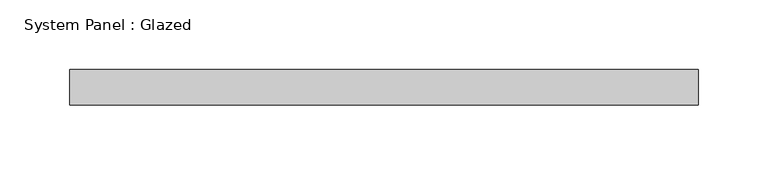
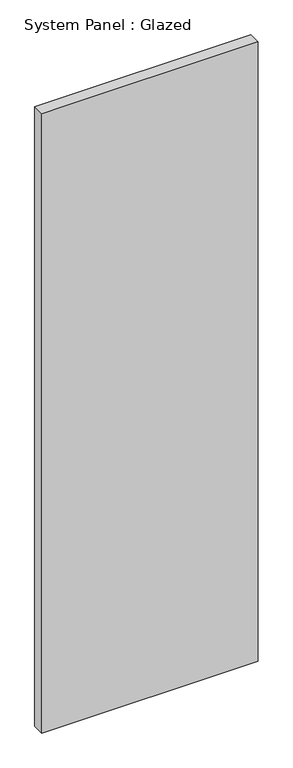
"""IFC4 building model written with IfcOpenShell, lengths in millimetres: plate geometry, System Panel : Glazed."""

from ifc_helpers import new_model, si_unit, origin, origin_with_axes, place, context, project, spatial, polyline, outline, extrude, source, transform, mapped, element, save


def system_panel_glazed_2348052a(model_context):
    return source(origin(), model_context, "Body", "SweptSolid", [
        extrude(outline(polyline([(225.425, 19.05), (-225.425, 19.05), (-225.425, 44.45), (225.425, 44.45), (225.425, 19.05)])), origin_with_axes(), (0.0, 0.0, 1.0), 1365.2228074),
    ])


if __name__ == "__main__":
    model = new_model("IFC4")
    model_context = context("Model", 3, world=origin())
    ifc_project = project(units=[si_unit("LENGTHUNIT", "METRE", prefix="MILLI")], contexts=[model_context])
    site = spatial("IfcSite", under=ifc_project)
    building = spatial("IfcBuilding", under=site)
    placement = place(None, origin())
    system_panel_glazed_shape = system_panel_glazed_2348052a(model_context)
    element("IfcPlate", 1, ObjectType="System Panel : Glazed", at=placement, inside=building, context=model_context, shape_type="MappedRepresentation", body=[
        mapped(system_panel_glazed_shape, transform((0.0, 0.0, 0.0), x_axis=(1.0, 0.0, 0.0), y_axis=(0.0, 1.0, 0.0), z_axis=(0.0, 0.0, 1.0))),
    ])
    save(model, "model.ifc")

# Revit data of these elements
# Type "System Panel : Glazed"
#   Construction Type Id = "GSP4R"
#   Analytic Construction = "1/8 in Pilkington single glazing"
#   Visual Light Transmittance = 0.9
#   Solar Heat Gain Coefficient = 0.86
#   Heat Transfer Coefficient (U) = 1.18115 BTU/(h·ft²·°F)
#   Define Thermal Properties by = 1
# Element 1 (IfcPlate, "System Panel : Glazed")
#   Materials on its faces: "Glass"
# Materials
#   "Glass": class "Glass", colour RGB 0 128 192, transparency 0.75, Description = "Soda Lime Glass", Cost = 0
